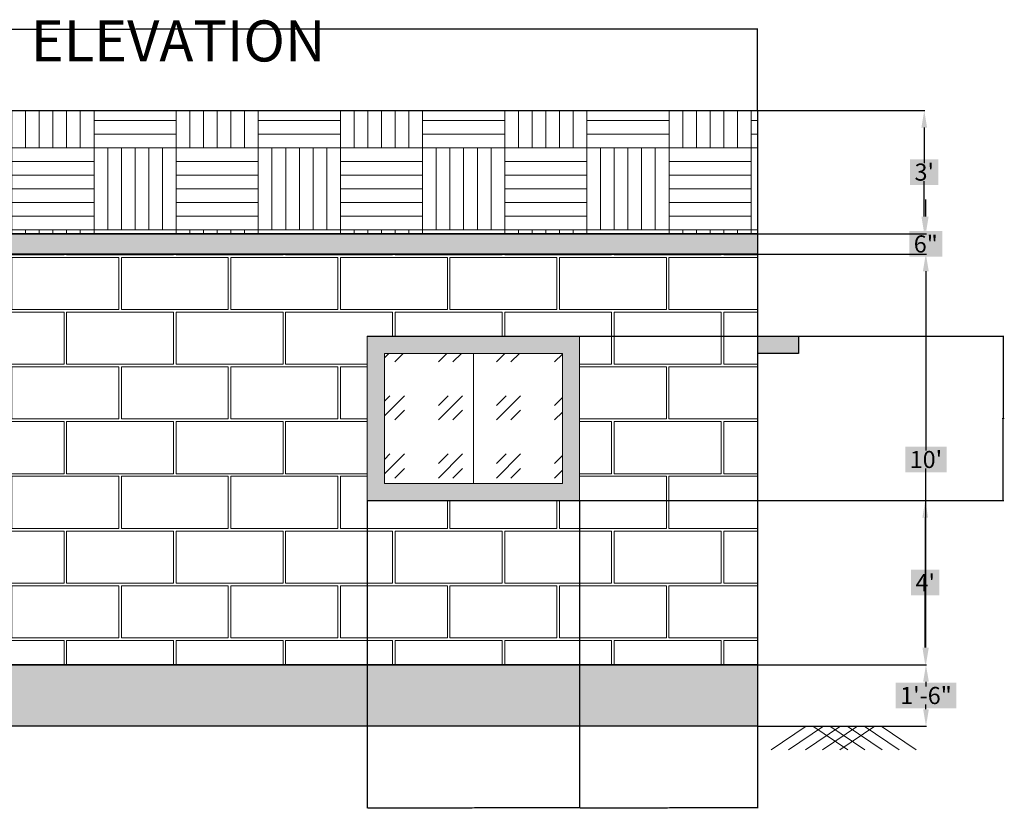
# Model space of a CAD drawing. Units: inches. Extents: x -128 to 854, y -395 to 398.
# Tile 60 of 61: x 567 to 854, y -395 to -165. Entities that reach past the tile are written whole.
import ezdxf

# ---------------------------------------------------------------- set-up
doc = ezdxf.new("R2010")
doc.units = ezdxf.units.IN
doc.header["$MEASUREMENT"] = 0
for name, color, linetype, lineweight in [('A-ANNO-DIMS', 2, 'Continuous', 18), ('A-ANNO-TITL', 7, 'Continuous', 25), ('A-ELEV', 3, 'Continuous', 25), ('A-ELEV-PATT', 8, 'Continuous', 13), ('A-GLAZ', 220, 'Continuous', 18), ('C-GRAD', 7, 'Continuous', 25), ('C-GRAD-PATT', 8, 'Continuous', 13)]:
    doc.layers.add(name, color=color, linetype=linetype, lineweight=lineweight)
doc.styles.get("Standard").update_dxf_attribs({"font": 'arial.ttf'})
doc.dimstyles.get("Standard").update_dxf_attribs({"dimtxt": 0.18, "dimasz": 0.18, "dimexe": 0.18, "dimexo": 0.0625, "dimgap": 0.09, "dimtad": 0, "dimtih": 1, "dimtoh": 1, "dimdec": 1, "dimzin": 0, "dimdsep": 46, "dimlunit": 4, "dimtxsty": 'Standard', "dimcen": 0.09, "dimclrd": 1, "dimclre": 2, "dimclrt": 6, "dimadec": 0, "dimazin": 0, "dimtfac": 1, "dimtdec": 1, "dimtofl": 0, "dimtmove": 0, "dimatfit": 3, "dimfxl": 1, "dimtfill": 2, "dimtfillclr": 3, "dimtolj": 1, "dimtzin": 0, "dimarcsym": 0})

# ---------------------------------------------------------------- blocks, each defined once
blk = doc.blocks.new('*D11')
at = {"layer": 'A-ANNO-DIMS', "color": 0, "lineweight": -2, "transparency": 16777216}
for p, q in [((782.34, -353.48), (831.69, -353.48)), ((831.51, -358.48), (831.51, -359.83)), ((831.51, -366.48), (831.51, -365.12)), ((782.34, -371.48), (831.69, -371.48))]:
    blk.add_line(p, q, dxfattribs=at)
at = {"layer": 'A-ANNO-DIMS', "color": 0, "transparency": 16777216}
for points in [[(830.68, -358.48), (832.35, -358.48), (831.51, -353.48)], [(830.68, -366.48), (832.35, -366.48), (831.51, -371.48)]]:
    blk.add_solid(points, dxfattribs=at)
at = {"layer": 'Defpoints', "color": 0, "transparency": 16777216}
for p in [(782.28, -353.48), (831.51, -353.48), (782.28, -371.48)]:
    blk.add_point(p, dxfattribs=at)
at = {"layer": 'A-ANNO-DIMS', "color": 0, "transparency": 16777216, "insert": (831.51, -362.48), "char_height": 5, "attachment_point": 5, "bg_fill": 1, "box_fill_scale": 1.25, "bg_fill_color": 3, "bg_fill_transparency": 0}
blk.add_mtext('\\A1;1\'-6"', dxfattribs=at)
blk = doc.blocks.new('*D12')
at = {"layer": 'A-ANNO-DIMS', "color": 0, "lineweight": -2, "transparency": 16777216}
for p, q in [((730.34, -305.48), (831.48, -305.48)), ((831.3, -310.48), (831.3, -326.89)), ((831.3, -348.48), (831.3, -332.07)), ((782.34, -353.48), (831.48, -353.48))]:
    blk.add_line(p, q, dxfattribs=at)
at = {"layer": 'A-ANNO-DIMS', "color": 0, "transparency": 16777216}
for points in [[(830.47, -310.48), (832.13, -310.48), (831.3, -305.48)], [(830.47, -348.48), (832.13, -348.48), (831.3, -353.48)]]:
    blk.add_solid(points, dxfattribs=at)
at = {"layer": 'Defpoints', "color": 0, "transparency": 16777216}
for p in [(730.28, -305.48), (831.3, -305.48), (782.28, -353.48)]:
    blk.add_point(p, dxfattribs=at)
at = {"layer": 'A-ANNO-DIMS', "color": 0, "transparency": 16777216, "insert": (831.3, -329.48), "char_height": 5, "attachment_point": 5, "bg_fill": 1, "box_fill_scale": 1.25, "bg_fill_color": 3, "bg_fill_transparency": 0}
blk.add_mtext("\\A1;4'", dxfattribs=at)
blk = doc.blocks.new('*D13')
at = {"layer": 'A-ANNO-DIMS', "color": 0, "lineweight": -2, "transparency": 16777216}
for p, q in [((782.34, -233.48), (831.68, -233.48)), ((831.5, -238.48), (831.5, -290.83)), ((831.5, -348.48), (831.5, -296.12)), ((782.34, -353.48), (831.68, -353.48))]:
    blk.add_line(p, q, dxfattribs=at)
at = {"layer": 'A-ANNO-DIMS', "color": 0, "transparency": 16777216}
for points in [[(830.66, -238.48), (832.33, -238.48), (831.5, -233.48)], [(830.66, -348.48), (832.33, -348.48), (831.5, -353.48)]]:
    blk.add_solid(points, dxfattribs=at)
at = {"layer": 'Defpoints', "color": 0, "transparency": 16777216}
for p in [(782.28, -233.48), (831.5, -233.48), (782.28, -353.48)]:
    blk.add_point(p, dxfattribs=at)
at = {"layer": 'A-ANNO-DIMS', "color": 0, "transparency": 16777216, "insert": (831.5, -293.48), "char_height": 5, "attachment_point": 5, "bg_fill": 1, "box_fill_scale": 1.25, "bg_fill_color": 3, "bg_fill_transparency": 0}
blk.add_mtext("\\A1;10'", dxfattribs=at)
blk = doc.blocks.new('*D14')
at = {"layer": 'A-ANNO-DIMS', "color": 0, "lineweight": -2, "transparency": 16777216}
for p, q in [((831.45, -222.48), (831.45, -217.48)), ((782.34, -227.48), (831.63, -227.48)), ((782.34, -233.48), (831.63, -233.48)), ((831.45, -238.48), (831.45, -243.48))]:
    blk.add_line(p, q, dxfattribs=at)
at = {"layer": 'A-ANNO-DIMS', "color": 0, "transparency": 16777216}
for points in [[(830.61, -222.48), (832.28, -222.48), (831.45, -227.48)], [(830.61, -238.48), (832.28, -238.48), (831.45, -233.48)]]:
    blk.add_solid(points, dxfattribs=at)
at = {"layer": 'Defpoints', "color": 0, "transparency": 16777216}
for p in [(782.28, -227.48), (831.45, -227.48), (782.28, -233.48)]:
    blk.add_point(p, dxfattribs=at)
at = {"layer": 'A-ANNO-DIMS', "color": 0, "transparency": 16777216, "insert": (831.45, -230.48), "char_height": 5, "attachment_point": 5, "bg_fill": 1, "box_fill_scale": 1.25, "bg_fill_color": 3, "bg_fill_transparency": 0}
blk.add_mtext('\\A1;6"', dxfattribs=at)
blk = doc.blocks.new('*D15')
at = {"layer": 'A-ANNO-DIMS', "color": 0, "lineweight": -2, "transparency": 16777216}
for p, q in [((782.34, -191.48), (831.19, -191.48)), ((831.01, -196.48), (831.01, -206.83)), ((831.01, -222.48), (831.01, -212.12)), ((782.34, -227.48), (831.19, -227.48))]:
    blk.add_line(p, q, dxfattribs=at)
at = {"layer": 'A-ANNO-DIMS', "color": 0, "transparency": 16777216}
for points in [[(830.18, -196.48), (831.84, -196.48), (831.01, -191.48)], [(830.18, -222.48), (831.84, -222.48), (831.01, -227.48)]]:
    blk.add_solid(points, dxfattribs=at)
at = {"layer": 'Defpoints', "color": 0, "transparency": 16777216}
for p in [(782.28, -191.48), (782.28, -227.48), (831.01, -227.48)]:
    blk.add_point(p, dxfattribs=at)
at = {"layer": 'A-ANNO-DIMS', "color": 0, "transparency": 16777216, "insert": (831.01, -209.48), "char_height": 5, "attachment_point": 5, "bg_fill": 1, "box_fill_scale": 1.25, "bg_fill_color": 3, "bg_fill_transparency": 0}
blk.add_mtext("\\A1;3'", dxfattribs=at)
blk = doc.blocks.new('*D133')
at = {"layer": 'A-ANNO-DIMS', "color": 2, "lineweight": -2, "transparency": 16777216}
for p, q in [((418.28, -191.41), (418.28, -167.5)), ((782.28, -191.41), (782.28, -167.5))]:
    blk.add_line(p, q, dxfattribs=at)
at = {"layer": 'A-ANNO-DIMS', "color": 1, "lineweight": -2, "transparency": 16777216}
for p, q in [((418.46, -167.68), (599.88, -167.68)), ((782.1, -167.68), (600.68, -167.68))]:
    blk.add_line(p, q, dxfattribs=at)
at = {"layer": 'A-ANNO-DIMS', "color": 1, "transparency": 16777216}
for points in [[(418.46, -167.65), (418.46, -167.71), (418.28, -167.68)], [(782.1, -167.65), (782.1, -167.71), (782.28, -167.68)]]:
    blk.add_solid(points, dxfattribs=at)
at = {"layer": 'Defpoints', "color": 0, "transparency": 16777216}
for p in [(782.28, -167.68), (418.28, -191.48), (782.28, -191.48)]:
    blk.add_point(p, dxfattribs=at)
at = {"layer": 'A-ANNO-DIMS', "color": 6, "transparency": 16777216, "insert": (600.28, -167.68), "char_height": 0.18, "attachment_point": 5, "bg_fill": 1, "box_fill_scale": 1.25, "bg_fill_color": 3, "bg_fill_transparency": 0}
blk.add_mtext('\\A1;30\'-4"', dxfattribs=at)
blk = doc.blocks.new('*D137')
at = {"layer": 'A-ANNO-DIMS', "color": 2, "lineweight": -2, "transparency": 16777216}
for p, q in [((730.28, -305.54), (730.28, -395.46)), ((782.28, -371.54), (782.28, -395.46))]:
    blk.add_line(p, q, dxfattribs=at)
at = {"layer": 'A-ANNO-DIMS', "color": 1, "lineweight": -2, "transparency": 16777216}
for p, q in [((730.46, -395.28), (755.95, -395.28)), ((782.1, -395.28), (756.61, -395.28))]:
    blk.add_line(p, q, dxfattribs=at)
at = {"layer": 'A-ANNO-DIMS', "color": 1, "transparency": 16777216}
for points in [[(730.46, -395.25), (730.46, -395.31), (730.28, -395.28)], [(782.1, -395.25), (782.1, -395.31), (782.28, -395.28)]]:
    blk.add_solid(points, dxfattribs=at)
at = {"layer": 'Defpoints', "color": 0, "transparency": 16777216}
for p in [(730.28, -305.48), (782.28, -371.48), (730.28, -395.28)]:
    blk.add_point(p, dxfattribs=at)
at = {"layer": 'A-ANNO-DIMS', "color": 6, "transparency": 16777216, "insert": (756.28, -395.28), "char_height": 0.18, "attachment_point": 5, "bg_fill": 1, "box_fill_scale": 1.25, "bg_fill_color": 3, "bg_fill_transparency": 0}
blk.add_mtext('\\A1;4\'-4"', dxfattribs=at)
blk = doc.blocks.new('*D138')
at = {"layer": 'A-ANNO-DIMS', "color": 2, "lineweight": -2, "transparency": 16777216}
for p, q in [((668.28, -305.54), (668.28, -395.46)), ((730.28, -305.54), (730.28, -395.46))]:
    blk.add_line(p, q, dxfattribs=at)
at = {"layer": 'A-ANNO-DIMS', "color": 1, "lineweight": -2, "transparency": 16777216}
for p, q in [((668.46, -395.28), (698.95, -395.28)), ((730.1, -395.28), (699.61, -395.28))]:
    blk.add_line(p, q, dxfattribs=at)
at = {"layer": 'A-ANNO-DIMS', "color": 1, "transparency": 16777216}
for points in [[(668.46, -395.25), (668.46, -395.31), (668.28, -395.28)], [(730.1, -395.25), (730.1, -395.31), (730.28, -395.28)]]:
    blk.add_solid(points, dxfattribs=at)
at = {"layer": 'Defpoints', "color": 0, "transparency": 16777216}
for p in [(668.28, -305.48), (730.28, -305.48), (730.28, -395.28)]:
    blk.add_point(p, dxfattribs=at)
at = {"layer": 'A-ANNO-DIMS', "color": 6, "transparency": 16777216, "insert": (699.28, -395.28), "char_height": 0.18, "attachment_point": 5, "bg_fill": 1, "box_fill_scale": 1.25, "bg_fill_color": 3, "bg_fill_transparency": 0}
blk.add_mtext('\\A1;5\'-2"', dxfattribs=at)
blk = doc.blocks.new('*D139')
at = {"layer": 'A-ANNO-DIMS', "color": 2, "lineweight": -2, "transparency": 16777216}
for p, q in [((668.34, -257.48), (854.26, -257.48)), ((668.34, -305.48), (854.26, -305.48))]:
    blk.add_line(p, q, dxfattribs=at)
at = {"layer": 'A-ANNO-DIMS', "color": 1, "lineweight": -2, "transparency": 16777216}
for p, q in [((854.08, -257.66), (854.08, -281.29)), ((854.08, -305.3), (854.08, -281.66))]:
    blk.add_line(p, q, dxfattribs=at)
at = {"layer": 'A-ANNO-DIMS', "color": 1, "transparency": 16777216}
for points in [[(854.05, -257.66), (854.11, -257.66), (854.08, -257.48)], [(854.05, -305.3), (854.11, -305.3), (854.08, -305.48)]]:
    blk.add_solid(points, dxfattribs=at)
at = {"layer": 'Defpoints', "color": 0, "transparency": 16777216}
for p in [(668.28, -257.48), (854.08, -257.48), (668.28, -305.48)]:
    blk.add_point(p, dxfattribs=at)
at = {"layer": 'A-ANNO-DIMS', "color": 6, "transparency": 16777216, "insert": (854.08, -281.48), "char_height": 0.18, "attachment_point": 5, "bg_fill": 1, "box_fill_scale": 1.25, "bg_fill_color": 3, "bg_fill_transparency": 0}
blk.add_mtext('\\A1;4\'-0"', dxfattribs=at)

msp = doc.modelspace()

# ---------------------------------------------------------------- hatches: boundary and pattern name
at = {"layer": 'A-ELEV-PATT'}
h = msp.add_hatch(dxfattribs=at)
h.set_pattern_fill('AR-PARQ1', color=256, scale=2)
h.set_pattern_definition([(90, (468.407, -10.41), (-24, 24), [24, -24]), (90, (472.407, -10.41), (-24, 24), [24, -24]), (90, (476.407, -10.41), (-24, 24), [24, -24]), (90, (480.407, -10.41), (-24, 24), [24, -24]), (90, (484.407, -10.41), (-24, 24), [24, -24]), (90, (488.407, -10.41), (-24, 24), [24, -24]), (90, (492.407, -10.41), (-24, 24), [24, -24]), (0, (468.407, 13.59), (24, -24), [24, -24]), (0, (468.407, 17.59), (24, -24), [24, -24]), (0, (468.407, 21.59), (24, -24), [24, -24]), (0, (468.407, 25.59), (24, -24), [24, -24]), (0, (468.407, 29.59), (24, -24), [24, -24]), (0, (468.407, 33.59), (24, -24), [24, -24]), (0, (468.407, 37.59), (24, -24), [24, -24])])
h.paths.add_polyline_path([(782.28, -227.48), (782.28, -191.48), (418.28, -191.48), (418.28, -227.48)])
h = msp.add_hatch(color=256, dxfattribs=at)
h.dxf.hatch_style = 1
h.paths.add_polyline_path([(418.28, -227.48), (418.28, -233.48), (782.28, -233.48), (782.28, -227.48)])
h.paths.add_polyline_path([(492.25, -257.48), (492.25, -353.48), (551.31, -353.48), (551.31, -257.48)])
h.paths.add_polyline_path([(546.31, -262.48), (546.31, -348.48), (497.25, -348.48), (497.25, -262.48)], flags=16)
h = msp.add_hatch(dxfattribs=at)
h.set_pattern_fill('AR-B816C', color=256, scale=2)
h.set_pattern_definition([(0, (468.407, -10.41), (16, 16), [31.25, -0.75]), (0, (452.407, -9.66), (16, 16), [31.25, -0.75]), (90, (468.407, -10.41), (-16, 16), [-16.75, 15.25]), (90, (467.657, -10.41), (-16, 16), [-16.75, 15.25])])
h.paths.add_polyline_path([(418.28, -353.48), (492.25, -353.48), (492.25, -257.48), (551.31, -257.48), (551.31, -353.48), (782.28, -353.48), (782.28, -233.48), (418.28, -233.48)])
h.paths.add_polyline_path([(668.28, -257.48), (730.28, -257.48), (730.28, -305.48), (668.28, -305.48)], flags=16)
h.paths.add_polyline_path([(673.28, -300.48), (673.28, -262.48), (725.28, -262.48), (725.28, -300.48)], flags=0)
h = msp.add_hatch(color=256, dxfattribs=at)
h.dxf.hatch_style = 1
h.paths.add_polyline_path([(406.28, -257.48), (406.28, -258.4), (406.28, -263.4), (418.28, -263.4), (418.28, -257.48)])
h.paths.add_polyline_path([(794.28, -262.48), (794.28, -257.48), (782.28, -257.48), (782.28, -262.48)])
h = msp.add_hatch(color=256, dxfattribs=at)
h.dxf.hatch_style = 1
h.paths.add_polyline_path([(668.28, -305.48), (730.28, -305.48), (730.28, -257.48), (668.28, -257.48)])
h.paths.add_polyline_path([(673.28, -262.48), (725.28, -262.48), (725.28, -300.48), (673.28, -300.48)], flags=16)
h = msp.add_hatch(dxfattribs=at)
h.set_pattern_fill('GOST_GLASS', color=256, scale=2)
h.set_pattern_definition([(45, (468.407, -10.41), (16.97056, -2e-15), [10, -14]), (45, (472.65, -10.41), (16.97056, -2e-15), [4, -20]), (45, (468.407, -6.168), (16.97056, -2e-15), [4, -20])])
h.paths.add_polyline_path([(699.28, -262.48), (673.28, -262.48), (673.28, -300.48), (699.28, -300.48)])
h.paths.add_polyline_path([(725.28, -262.48), (699.28, -262.48), (699.28, -300.48), (725.28, -300.48)])
h = msp.add_hatch(dxfattribs=at)
h.set_pattern_fill('AR-CONC', color=256, scale=2)
h.set_pattern_definition([(50, (468.407, -10.41), (14.3452, -1.25504), [1.5, -16.5]), (355, (468.407, -10.41), (-2.77503, 15.04384), [1.2, -13.2]), (100.4514, (469.602, -10.515), (11.57018, 13.7888), [1.2748, -14.02284]), (46.184, (468.407, -6.41), (21.3448, -3.3104), [2.25, -24.75]), (96.6356, (470.186, -6.686), (18.6932, 19.4824), [1.9122, -21.0343]), (351.184, (468.407, -6.41), (18.6932, 19.4824), [1.8, -19.8]), (21, (470.407, -7.41), (11.93814, -8.05238), [1.5, -16.5]), (326, (470.407, -7.41), (4.8663, 14.503), [1.2, -13.2]), (71.4514, (471.402, -8.081), (16.80445, 6.45062), [1.2748, -14.02284]), (37.5, (468.407, -10.4104), (0.243197, 6.657877), [0, -13.04, 0, -13.4, 0, -13.25]), (7.5, (468.407, -10.4104), (5.26139, 7.88823), [0, -7.64, 0, -12.74, 0, -5.05]), (327.5, (463.947, -10.4104), (10.67645, -0.4511), [0, -5, 0, -15.6, 0, -20.7]), (317.5, (461.947, -10.41), (11.66372, 2.0021), [0, -6.5, 0, -10.36, 0, -14.7])])
h.paths.add_polyline_path([(418.28, -353.48), (418.28, -371.48), (492.25, -371.48), (492.25, -353.48)])
h.paths.add_polyline_path([(782.28, -371.48), (782.28, -353.48), (551.31, -353.48), (551.31, -371.48)])
at = {"layer": 'C-GRAD-PATT'}
h = msp.add_hatch(dxfattribs=at)
h.set_pattern_fill('ANSI31', color=256, scale=22.43157, angle=349.1104, style=0)
h.paths.add_polyline_path([(794.64, -371.48), (819.62, -371.48), (809.39, -378.4), (784.41, -378.4)])
h = msp.add_hatch(dxfattribs=at)
h.set_pattern_fill('ANSI31', color=256, scale=22.43157, angle=100.8896, style=0)
h.paths.add_polyline_path([(794.64, -371.48), (819.62, -371.48), (829.85, -378.4), (804.87, -378.4)])

# ---------------------------------------------------------------- linework, layer by layer
at = {"layer": 'A-ELEV'}
for p, q in [((782.28, -257.48), (794.28, -257.48)), ((794.28, -257.48), (794.28, -262.48)), ((794.28, -262.48), (782.28, -262.48))]:
    msp.add_line(p, q, dxfattribs=at)
for points in [[(418.28, -191.48), (782.28, -191.48), (782.28, -227.48), (418.28, -227.48)], [(418.28, -227.48), (782.28, -227.48), (782.28, -233.48), (418.28, -233.48)], [(418.28, -233.48), (782.28, -233.48), (782.28, -353.48), (418.28, -353.48)], [(418.28, -353.48), (782.28, -353.48), (782.28, -371.48), (418.28, -371.48)]]:
    msp.add_lwpolyline(points, close=True, dxfattribs=at)
at = {"layer": 'A-GLAZ'}
msp.add_line((699.28, -262.48), (699.28, -300.48), dxfattribs=at)
for points in [[(668.28, -257.48), (730.28, -257.48), (730.28, -305.48), (668.28, -305.48)], [(673.28, -262.48), (725.28, -262.48), (725.28, -300.48), (673.28, -300.48)]]:
    msp.add_lwpolyline(points, close=True, dxfattribs=at)
at = {"layer": 'C-GRAD'}
msp.add_line((782.28, -371.48), (830.28, -371.48), dxfattribs=at)

# ---------------------------------------------------------------- texts
at = {"layer": 'A-ANNO-TITL'}
msp.add_text('ELEVATION', height=12, dxfattribs=at).set_placement((569.93, -177.13))

# ---------------------------------------------------------------- dimensions: what is measured, and where the dimension line sits
at = {"layer": 'A-ANNO-DIMS'}
for base, p1, p2, picture, middle in [((782.28, -167.68), (418.28, -191.48), (782.28, -191.48), '*D133', (600.28, -167.68)), ((730.28, -395.28), (668.28, -305.48), (730.28, -305.48), '*D138', (699.28, -395.28)), ((730.28, -395.28), (782.28, -371.48), (730.28, -305.48), '*D137', (756.28, -395.28))]:
    dim = msp.add_linear_dim(base=base, p1=p1, p2=p2, dimstyle='Standard', override={"dimdec": 1, "dimlfac": 1, "dimrnd": 0, "dimzin": 1, "dimdsep": 46, "dimlunit": 4, "dimfrac": 2}, dxfattribs=at)
    dim.commit()
    dim.dimension.update_dxf_attribs({"geometry": picture, "text_midpoint": middle})
for base, p1, p2, override, picture, middle in [((831.01, -227.48), (782.28, -191.48), (782.28, -227.48), {"dimtxt": 5, "dimasz": 5, "dimclrd": 0, "dimclre": 0, "dimclrt": 0}, '*D15', (831.01, -209.48)), ((831.45, -227.48), (782.28, -233.48), (782.28, -227.48), {"dimtxt": 5, "dimasz": 5, "dimclrd": 0, "dimclre": 0, "dimclrt": 0}, '*D14', (831.45, -230.48)), ((831.5, -233.48), (782.28, -353.48), (782.28, -233.48), {"dimtxt": 5, "dimasz": 5, "dimclrd": 0, "dimclre": 0, "dimclrt": 0}, '*D13', (831.5, -293.48)), ((854.08, -257.48), (668.28, -305.48), (668.28, -257.48), {"dimdec": 1, "dimlfac": 1, "dimrnd": 0, "dimzin": 1, "dimdsep": 46, "dimlunit": 4, "dimfrac": 2}, '*D139', (854.08, -281.48)), ((831.3, -305.48), (782.28, -353.48), (730.28, -305.48), {"dimtxt": 5, "dimasz": 5, "dimclrd": 0, "dimclre": 0, "dimclrt": 0}, '*D12', (831.3, -329.48)), ((831.51, -353.48), (782.28, -371.48), (782.28, -353.48), {"dimtxt": 5, "dimasz": 5, "dimclrd": 0, "dimclre": 0, "dimclrt": 0}, '*D11', (831.51, -362.48))]:
    dim = msp.add_linear_dim(base=base, p1=p1, p2=p2, angle=90, dimstyle='Standard', override=override, dxfattribs=at)
    dim.commit()
    dim.dimension.update_dxf_attribs({"geometry": picture, "text_midpoint": middle})

doc.saveas('drawing.dxf')
